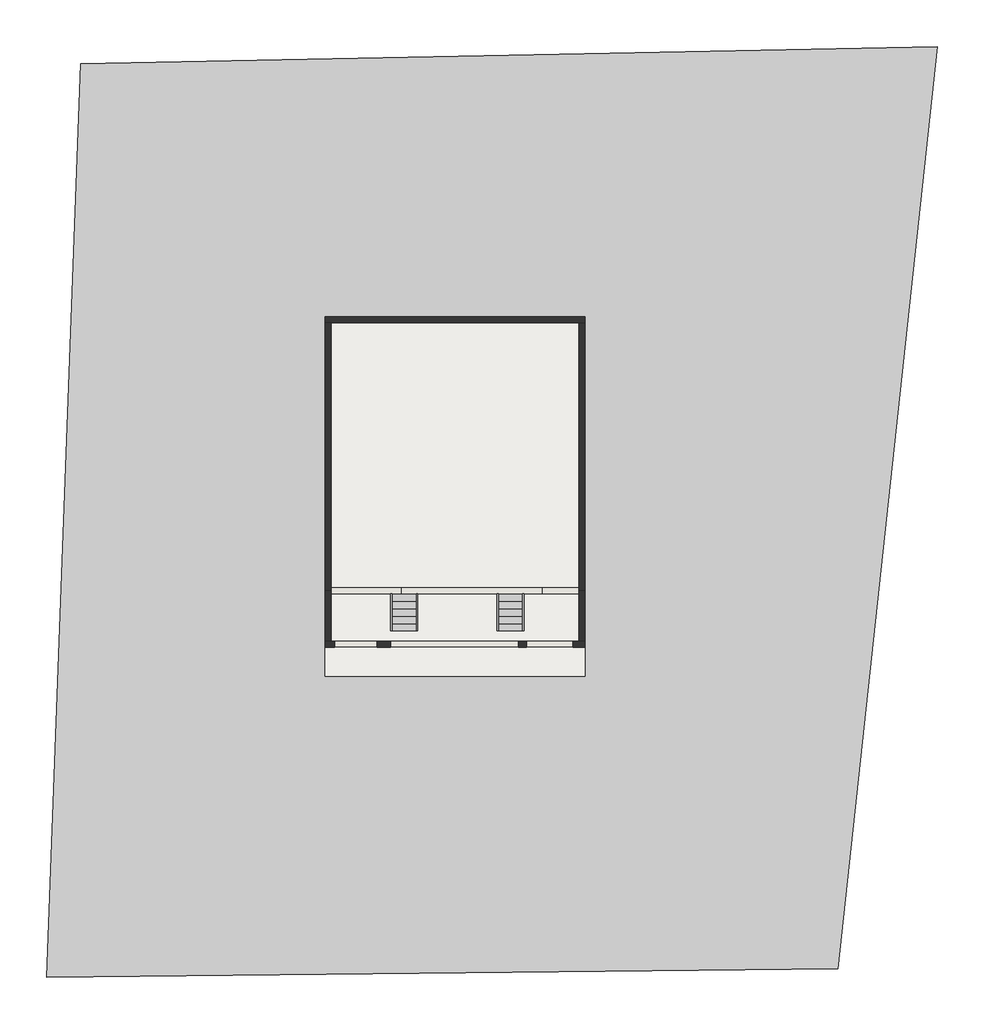
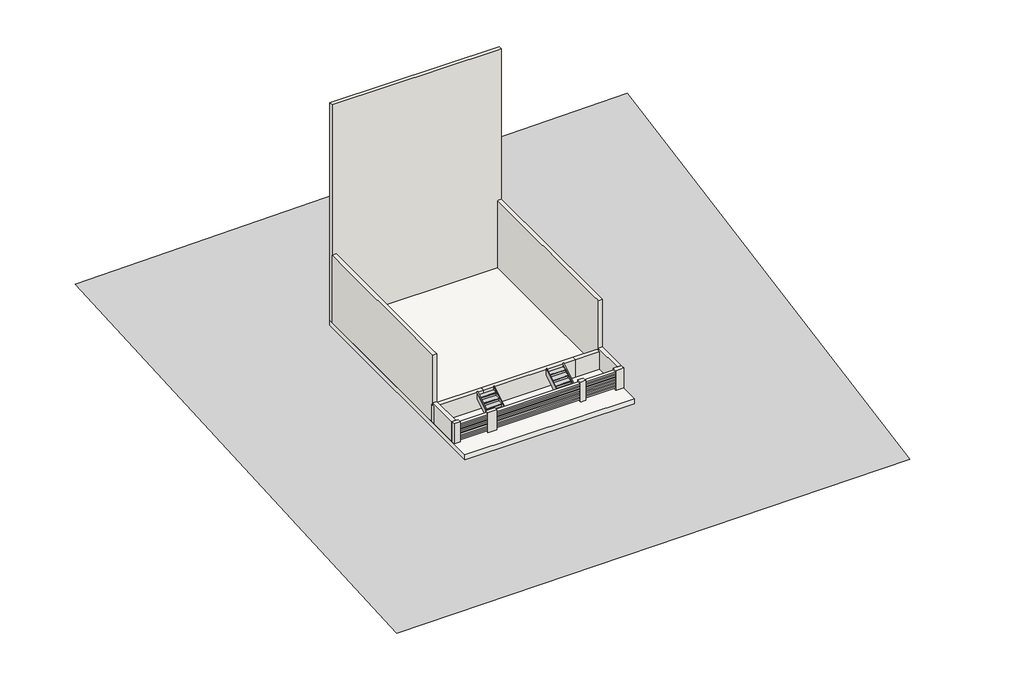
# One storey: 13 walls, 4 members, 2 stair flights, 1 proxy, 1 slab.
"""IFC4 building model written with IfcOpenShell, lengths in millimetres."""

from ifc_helpers import new_model, si_unit, frame, origin, place, context, project, spatial, polyline, outline, extrude, faceted_brep, triangles, transform, mapped, element, save
from components import stair_flight_369be8b3, stair_flight_a146ff17, walls_1_walls_1_ee36d61b

model = new_model("IFC4")

# Units and contexts
model_context = context("Model", 3, world=origin())
ifc_project = project(units=[si_unit("LENGTHUNIT", "METRE", prefix="MILLI")], contexts=[model_context])

# Site, building, storey
site = spatial("IfcSite", under=ifc_project)
building = spatial("IfcBuilding", under=site)
storey = spatial("IfcBuildingStorey", under=building, Elevation=-1066.8)

# Proxy
placement = place(None, origin())
element("IfcBuildingElementProxy", 1, Name="Building Element Proxy", at=placement, inside=storey, context=model_context, shape_type="Tessellation", body=[
    triangles([(-15502.9630188, 18397.3619293, -1422.3999516), (-16780.8489716, -15892.5834229, -1422.3999516), (12930.0037903, -15573.1122253, -1422.3999516), (16657.171637, 19036.3043243, -1422.3999516)], [[1, 2, 3], [3, 4, 1]], closed=False),
])

# Members
element("IfcMember", 2, ObjectType="Stringer - 2\" Width", at=placement, inside=storey, context=model_context, shape_type="SweptSolid", body=[
    extrude(outline(polyline([(-2893.1217987, -1066.8), (-2893.1217987, -851.7893563), (-1496.1217987, 37.2106437), (-1496.1217987, -324.0717005), (-2663.2662693, -1066.8), (-2893.1217987, -1066.8)])), frame((-3861.358803, 0.0, 0.0), z_axis=(1.0, 0.0, 0.0), x_axis=(0.0, 1.0, 0.0)), (0.0, 0.0, 1.0), 50.8),
])
element("IfcMember", 3, ObjectType="Stringer - 2\" Width", at=placement, inside=storey, context=model_context, shape_type="SweptSolid", body=[
    extrude(outline(polyline([(-2893.1217987, -1066.8), (-2893.1217987, -851.7893563), (-1496.1217987, 37.2106437), (-1496.1217987, -324.0717005), (-2663.2662693, -1066.8), (-2893.1217987, -1066.8)])), frame((-2896.158803, 0.0, 0.0), z_axis=(1.0, 0.0, 0.0), x_axis=(0.0, 1.0, 0.0)), (0.0, 0.0, 1.0), 50.8),
])
element("IfcMember", 4, ObjectType="Stringer - 2\" Width", at=placement, inside=storey, context=model_context, shape_type="SweptSolid", body=[
    extrude(outline(polyline([(-2893.1217987, -1066.8), (-2893.1217987, -851.7893563), (-1496.1217987, 37.2106437), (-1496.1217987, -324.0717005), (-2663.2662693, -1066.8), (-2893.1217987, -1066.8)])), frame((126.441197, 0.0, 0.0), z_axis=(1.0, 0.0, 0.0), x_axis=(0.0, 1.0, 0.0)), (0.0, 0.0, 1.0), 50.8),
])
element("IfcMember", 5, ObjectType="Stringer - 2\" Width", at=placement, inside=storey, context=model_context, shape_type="SweptSolid", body=[
    extrude(outline(polyline([(-2893.1217987, -1066.8), (-2893.1217987, -851.7893563), (-1496.1217987, 37.2106437), (-1496.1217987, -324.0717005), (-2663.2662693, -1066.8), (-2893.1217987, -1066.8)])), frame((1091.641197, 0.0, 0.0), z_axis=(1.0, 0.0, 0.0), x_axis=(0.0, 1.0, 0.0)), (0.0, 0.0, 1.0), 50.8),
])

# Slab
element("IfcSlab", 6, ObjectType="Generic - 12\"", at=placement, inside=storey, context=model_context, shape_type="SweptSolid", body=[
    extrude(outline(polyline([(3431.5769214, -4582.2217987), (-6322.0230786, -4582.2217987), (-6322.0230786, 8902.3535822), (3431.5769214, 8902.3535822), (3431.5769214, -4582.2217987)])), frame((0.0, 0.0, -1371.6), z_axis=(0.0, 0.0, 1.0), x_axis=(1.0, 0.0, 0.0)), (0.0, 0.0, 1.0), 304.8),
])

# Stair flights
stair_flight_shape = stair_flight_369be8b3(model_context)
element("IfcStairFlight", 7, ObjectType="2\" Tread 1\" Nosing 1/4\" Riser", at=placement, inside=storey, context=model_context, shape_type="MappedRepresentation", body=[
    mapped(stair_flight_shape, transform((0.0, 0.0, 0.0), x_axis=(1.0, 0.0, 0.0), y_axis=(0.0, 1.0, 0.0), z_axis=(0.0, 0.0, 1.0))),
])
stair_flight_2_shape = stair_flight_a146ff17(model_context)
element("IfcStairFlight", 8, ObjectType="2\" Tread 1\" Nosing 1/4\" Riser", at=placement, inside=storey, context=model_context, shape_type="MappedRepresentation", body=[
    mapped(stair_flight_2_shape, transform((0.0, 0.0, 0.0), x_axis=(1.0, 0.0, 0.0), y_axis=(0.0, 1.0, 0.0), z_axis=(0.0, 0.0, 1.0))),
])

# Walls
element("IfcWall", 9, ObjectType="9\"", at=placement, inside=storey, context=model_context, shape_type="Brep", body=[
    faceted_brep([(-6322.0230786, 8673.7535822, 12192.0), (-6322.0230786, 8673.7535822, 12000.3983116), (-6322.0230786, 8673.7535822, 3048.0), (-6322.0230786, 8673.7535822, -1066.8), (-6093.4230786, 8673.7535822, -1066.8), (3202.9769214, 8673.7535822, -1066.8), (3431.5769214, 8673.7535822, -1066.8), (3431.5769214, 8673.7535822, 3048.0), (3431.5769214, 8673.7535822, 12192.0), (3202.9769214, 8673.7535822, 12192.0), (-6322.0230786, 8902.3535822, -1066.8), (-6322.0230786, 8902.3535822, 12192.0), (3431.5769214, 8902.3535822, 12192.0), (3431.5769214, 8902.3535822, -1066.8)], [[[0, 1, 2, 3, 4, 5, 6, 7, 8, 9]], [[10, 11, 12, 13]], [[6, 5, 4, 3, 10, 13]], [[0, 9, 8, 12, 11]], [[0, 11, 10, 3, 2, 1]], [[6, 13, 12, 8, 7]]]),
])
element("IfcWall", 10, ObjectType="9\"", at=placement, inside=storey, context=model_context, shape_type="Brep", body=[
    faceted_brep([(-6322.0230786, -1496.1217235, -1066.8), (-6093.4230786, -1496.1217235, -1066.8), (-3475.4457527, -1496.1217235, -1066.8), (-3475.4457527, -1496.1217235, 0.0), (-6093.4230786, -1496.1217235, 0.0), (-6322.0230786, -1496.1217235, 0.0), (-6322.0230786, -1267.5217235, -1066.8), (-6322.0230786, -1267.5217235, 0.0), (-6093.4230786, -1267.5217235, 0.0), (-3475.4457527, -1267.5217235, 0.0), (-3475.4457527, -1267.5217235, -1066.8), (-6093.4230786, -1267.5217235, -1066.8), (-6322.0230786, -1381.8217235, 0.0)], [[[0, 1, 2, 3, 4, 5]], [[6, 7, 8, 9, 10, 11]], [[2, 1, 0, 6, 11, 10]], [[3, 2, 10, 9]], [[5, 4, 3, 9, 8, 7, 12]], [[0, 5, 12, 7, 6]]]),
])
element("IfcWall", 11, ObjectType="9\"", at=placement, inside=storey, context=model_context, shape_type="Brep", body=[
    faceted_brep([(3431.5769214, -1267.5217235, -1066.8), (3202.9769214, -1267.5217235, -1066.8), (1809.4464028, -1267.5217235, -1066.8), (1809.4464028, -1267.5217235, 0.0), (3202.9769214, -1267.5217235, 0.0), (3431.5769214, -1267.5217235, 0.0), (3431.5769214, -1496.1217235, -1066.8), (3431.5769214, -1496.1217235, 0.0), (3202.9769214, -1496.1217235, 0.0), (1809.4464028, -1496.1217235, 0.0), (1809.4464028, -1496.1217235, -1066.8), (3202.9769214, -1496.1217235, -1066.8), (3431.5769214, -1381.8217235, 0.0)], [[[0, 1, 2, 3, 4, 5]], [[6, 7, 8, 9, 10, 11]], [[2, 1, 0, 6, 11, 10]], [[3, 2, 10, 9]], [[5, 4, 3, 9, 8, 7, 12]], [[0, 5, 12, 7, 6]]]),
])
element("IfcWall", 12, ObjectType="9\"", at=placement, inside=storey, context=model_context, shape_type="SweptSolid", body=[
    extrude(outline(polyline([(1809.4464028, -1496.1217987), (-3475.4457527, -1496.1217987), (-3475.4457527, -1267.5217987), (1809.4464028, -1267.5217987), (1809.4464028, -1496.1217987)])), frame((0.0, 0.0, -1066.8), z_axis=(0.0, 0.0, 1.0), x_axis=(1.0, 0.0, 0.0)), (0.0, 0.0, 1.0), 1066.8),
])
element("IfcWall", 13, ObjectType="9\"", at=placement, inside=storey, context=model_context, shape_type="Brep", body=[
    faceted_brep([(-6322.0230786, 8673.7535822, -1066.8), (-6322.0230786, -1267.5217235, -1066.8), (-6322.0230786, -1267.5217235, 0.0), (-6322.0230786, -1381.8217235, 0.0), (-6322.0230786, -1381.8217235, 152.4), (-6322.0230786, -1381.8217235, 3048.0), (-6322.0230786, -394.0464931, 3048.0), (-6322.0230786, 8673.7535822, 3048.0), (-6093.4230786, 8673.7535822, -1066.8), (-6093.4230786, 8673.7535822, 3048.0), (-6093.4230786, -394.0464931, 3048.0), (-6093.4230786, -1038.9217235, 3048.0), (-6093.4230786, -1267.5217235, 3048.0), (-6093.4230786, -1381.8217235, 3048.0), (-6093.4230786, -1381.8217235, 152.4), (-6093.4230786, -1381.8217235, 0.0), (-6093.4230786, -1267.5217235, 0.0), (-6093.4230786, -1267.5217235, -1066.8)], [[[0, 1, 2, 3, 4, 5, 6, 7]], [[8, 9, 10, 11, 12, 13, 14, 15, 16, 17]], [[1, 0, 8, 17]], [[7, 6, 5, 13, 12, 11, 10, 9]], [[0, 7, 9, 8]], [[5, 4, 3, 15, 14, 13]], [[15, 3, 2, 16]], [[2, 1, 17, 16]]]),
])
element("IfcWall", 14, ObjectType="9\"", at=placement, inside=storey, context=model_context, shape_type="Brep", body=[
    faceted_brep([(3202.9769214, 8673.7535822, -1066.8), (3202.9769214, -1267.5217235, -1066.8), (3202.9769214, -1267.5217235, 0.0), (3202.9769214, -1381.8217235, 0.0), (3202.9769214, -1381.8217235, 152.4), (3202.9769214, -1381.8217235, 3048.0), (3202.9769214, -1267.5217235, 3048.0), (3202.9769214, -1038.9217235, 3048.0), (3202.9769214, -394.0464931, 3048.0), (3202.9769214, 8673.7535822, 3048.0), (3431.5769214, 8673.7535822, -1066.8), (3431.5769214, 8673.7535822, 3048.0), (3431.5769214, -394.0464931, 3048.0), (3431.5769214, -1381.8217235, 3048.0), (3431.5769214, -1381.8217235, 152.4), (3431.5769214, -1381.8217235, 0.0), (3431.5769214, -1267.5217235, 0.0), (3431.5769214, -1267.5217235, -1066.8)], [[[0, 1, 2, 3, 4, 5, 6, 7, 8, 9]], [[10, 11, 12, 13, 14, 15, 16, 17]], [[1, 0, 10, 17]], [[9, 8, 7, 6, 5, 13, 12, 11]], [[0, 9, 11, 10]], [[5, 4, 3, 15, 14, 13]], [[15, 3, 2, 16]], [[2, 1, 17, 16]]]),
])
element("IfcWall", 15, ObjectType="9\"", at=placement, inside=storey, context=model_context, shape_type="SweptSolid", body=[
    extrude(outline(polyline([(-4378.9230786, -3274.1217987), (-3861.358803, -3274.1217987), (-3861.358803, -3502.7217987), (-4378.9230786, -3502.7217987), (-4378.9230786, -3274.1217987)])), frame((0.0, 0.0, -1066.8), z_axis=(0.0, 0.0, 1.0), x_axis=(1.0, 0.0, 0.0)), (0.0, 0.0, 1.0), 1219.2),
])
element("IfcWall", 16, ObjectType="9\"", at=placement, inside=storey, context=model_context, shape_type="Brep", body=[
    faceted_brep([(-6322.0230786, -3502.7217987, -1066.8), (-5965.6185982, -3502.7217987, -1066.8), (-5965.6185982, -3502.7217987, 152.4), (-6322.0230786, -3502.7217987, 152.4), (-6322.0230786, -3274.1217987, -1066.8), (-6322.0230786, -3274.1217987, 152.4), (-6093.4230786, -3274.1217987, 152.4), (-5965.6185982, -3274.1217987, 152.4), (-5965.6185982, -3274.1217987, -1066.8), (-6093.4230786, -3274.1217987, -1066.8)], [[[0, 1, 2, 3]], [[4, 5, 6, 7, 8, 9]], [[1, 0, 4, 9, 8]], [[2, 1, 8, 7]], [[3, 2, 7, 6, 5]], [[0, 3, 5, 4]]]),
])
element("IfcWall", 17, ObjectType="9\"", at=placement, inside=storey, context=model_context, shape_type="Brep", body=[
    faceted_brep([(3431.5769214, -3274.1217987, -1066.8), (3202.9769214, -3274.1217987, -1066.8), (2974.3769214, -3274.1217987, -1066.8), (2974.3769214, -3274.1217987, 152.4), (3202.9769214, -3274.1217987, 152.4), (3431.5769214, -3274.1217987, 152.4), (3431.5769214, -3502.7217987, -1066.8), (3431.5769214, -3502.7217987, 152.4), (2974.3769214, -3502.7217987, 152.4), (2974.3769214, -3502.7217987, -1066.8)], [[[0, 1, 2, 3, 4, 5]], [[6, 7, 8, 9]], [[2, 1, 0, 6, 9]], [[3, 2, 9, 8]], [[5, 4, 3, 8, 7]], [[0, 5, 7, 6]]]),
])
element("IfcWall", 18, ObjectType="9\"", at=placement, inside=storey, context=model_context, shape_type="SweptSolid", body=[
    extrude(outline(polyline([(1244.041197, -3502.7217987), (939.241197, -3502.7217987), (939.241197, -3274.1217987), (1244.041197, -3274.1217987), (1244.041197, -3502.7217987)])), frame((0.0, 0.0, -1066.8), z_axis=(0.0, 0.0, 1.0), x_axis=(1.0, 0.0, 0.0)), (0.0, 0.0, 1.0), 1219.2),
])
element("IfcWall", 19, ObjectType="9\"", at=placement, inside=storey, context=model_context, shape_type="SweptSolid", body=[
    extrude(outline(polyline([(-1496.1217235, -1066.8), (-3274.1217987, -1066.8), (-3274.1217987, 152.4), (-1381.8217235, 152.4), (-1381.8217235, 0.0), (-1496.1217235, 0.0), (-1496.1217235, -1066.8)])), frame((-6322.0230786, 0.0, 0.0), z_axis=(1.0, 0.0, 0.0), x_axis=(0.0, 1.0, 0.0)), (0.0, 0.0, 1.0), 228.6),
])
element("IfcWall", 20, ObjectType="9\"", at=placement, inside=storey, context=model_context, shape_type="SweptSolid", body=[
    extrude(outline(polyline([(-1496.1217235, -1066.8), (-3274.1217987, -1066.8), (-3274.1217987, 152.4), (-1381.8217235, 152.4), (-1381.8217235, 0.0), (-1496.1217235, 0.0), (-1496.1217235, -1066.8)])), frame((3202.9769214, 0.0, 0.0), z_axis=(1.0, 0.0, 0.0), x_axis=(0.0, 1.0, 0.0)), (0.0, 0.0, 1.0), 228.6),
])
walls_1_walls_1_shape = walls_1_walls_1_ee36d61b(model_context)
element("IfcWall", 21, ObjectType="Walls 1 : Walls 1", at=placement, inside=storey, context=model_context, shape_type="MappedRepresentation", body=[
    mapped(walls_1_walls_1_shape, transform((0.0, 0.0, 0.0), x_axis=(1.0, 0.0, 0.0), y_axis=(0.0, 1.0, 0.0), z_axis=(0.0, 0.0, 1.0))),
])

save(model, "model.ifc")

# Revit data of these elements
# Type "Generic - 12\""
#   Assembly Code = "B1010"
#   Function = 0
#   Layers, outside or top first: 1' - 0" no material (function 1)
# Type "9\""
#   Assembly Code = "B2010"
#   Layers, outside or top first: 0' - 9" no material (function 1)
# Element 1 (IfcBuildingElementProxy)
#   Material = none
#   Phase Created = New Construction
# Elements 2, 3, 4, 5 (IfcMember, "Stringer - 2\" Width")
#   Phase Created = New Construction
# Element 6 (IfcSlab, "Generic - 12\"")
#   Height Offset From Level = 0' - 0"
#   Phase Created = New Construction
#   Materials on its faces: "Default Floor"
# Elements 7, 8 (IfcStairFlight, "2\" Tread 1\" Nosing 1/4\" Riser")
#   Phase Created = New Construction
# Element 9 (IfcWall, "9\"")
#   Top Offset = 0' - 0"
#   Base Offset = 0' - 0"
#   wall height = 43' - 6"
#   Phase Created = New Construction
#   Top Constraint = FOURTH FLOOR
#   Materials on its faces: "Default Wall", "1 wall"
# Elements 10, 11 (IfcWall, "9\"")
#   Top Offset = 0' - 0"
#   Base Offset = 0' - 0"
#   Unconnected Height = 3' - 6"
#   wall height = 3' - 6"
#   Phase Created = New Construction
#   Materials on its faces: "Default Wall", "1 wall"
# Element 12 (IfcWall, "9\"")
#   Top Offset = 0' - 0"
#   Base Offset = 0' - 0"
#   Unconnected Height = 3' - 6"
#   wall height = 3' - 6"
#   Phase Created = New Construction
#   Materials on its faces: "Default Wall"
# Elements 13, 14 (IfcWall, "9\"")
#   Top Offset = 0' - 0"
#   Base Offset = 0' - 0"
#   wall height = 13' - 6"
#   Phase Created = New Construction
#   Top Constraint = FIRST FLOOR
#   Materials on its faces: "Default Wall", "1 wall"
# Elements 15, 17, 18, 19, 20 (IfcWall, "9\"")
#   Top Offset = 0' - 0"
#   Base Offset = 0' - 0"
#   Unconnected Height = 4' - 0"
#   wall height = 4' - 0"
#   Phase Created = New Construction
#   Materials on its faces: "Default Wall", "1 wall"
# Element 16 (IfcWall, "9\"")
#   Top Offset = 0' - 0"
#   Base Offset = 0' - 0"
#   Unconnected Height = 4' - 0"
#   wall height = 4' - 0"
#   Phase Created = New Construction
#   Materials on its faces: "1 wall", "Default Wall"
# Element 21 (IfcWall, "Walls 1 : Walls 1")
#   Phase Created = New Construction
#   Materials on its faces: "Default Wall"
# Materials
#   "Default Floor": colour RGB 128 128 128, transparency 0, Cost = 0
#   "Default Wall": colour RGB 128 128 128, transparency 0, Cost = 0
#   "1 wall": class "Generic", colour RGB 244 245 241, transparency 0, Cost = 0
